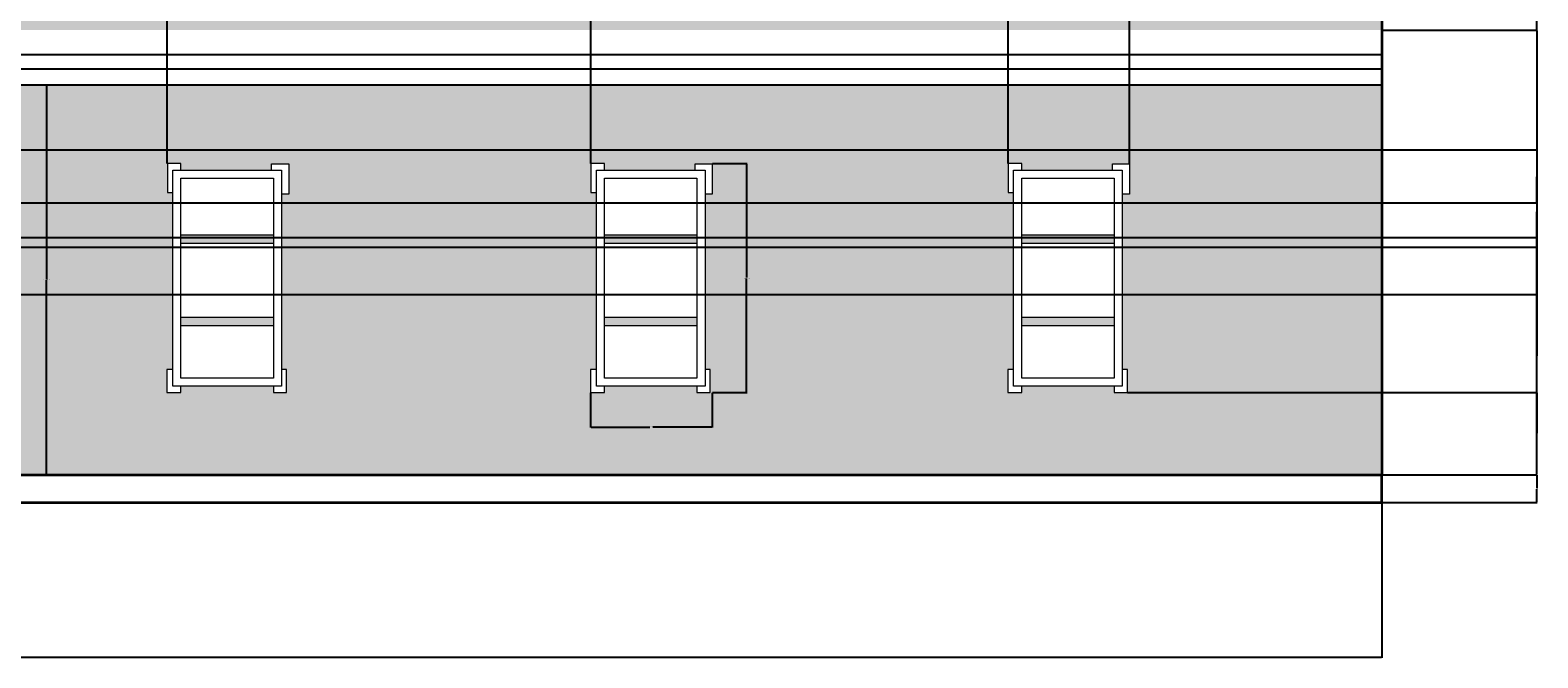
# Model space of a CAD drawing. Units: inches. Extents: x -46 to 1209, y 110 to 778.
# Tile 4 of 5: x 652 to 1209, y 110 to 342. Entities that reach past the tile are written whole.
import ezdxf

# ---------------------------------------------------------------- set-up
doc = ezdxf.new("R2010")
doc.units = ezdxf.units.IN
doc.header["$MEASUREMENT"] = 0
for name, color, linetype, lineweight in [('A-ANNO-DIMS', 2, 'Continuous', 18), ('A-ELEV-BASE', 7, 'Continuous', 35), ('A-GLAZ', 4, 'Continuous', 20), ('A-GLAZ-PATT', 9, 'Continuous', 13), ('A-WALL', 7, 'Continuous', 35), ('A-WALL-PATT', 252, 'Continuous', 13), ('A-WALL-TRIM', 42, 'Continuous', 25)]:
    doc.layers.add(name, color=color, linetype=linetype, lineweight=lineweight)
doc.styles.get("Standard").update_dxf_attribs({"font": 'arial.ttf'})
doc.dimstyles.get("Standard").update_dxf_attribs({"dimtxt": 0.18, "dimasz": 0.18, "dimexe": 0.18, "dimexo": 0.0625, "dimgap": 0.09, "dimtad": 0, "dimtih": 1, "dimtoh": 1, "dimdec": 4, "dimzin": 0, "dimdsep": 46, "dimtxsty": 'Standard', "dimcen": 0.09, "dimadec": 0, "dimazin": 0, "dimtfac": 1, "dimtdec": 4, "dimtofl": 0, "dimtmove": 0, "dimatfit": 3, "dimfxl": 1, "dimtolj": 1, "dimtzin": 0, "dimarcsym": 0})

# ---------------------------------------------------------------- blocks, each defined once
blk = doc.blocks.new('WIN-TALL-3-LIGHT')
for p, q in [((5.17, 84.79), (0.14, 84.79)), ((0.14, 84.79), (0.14, 74.08)), ((5.17, 82.37), (5.17, 84.79)), ((38.71, 82.37), (38.71, 84.69)), ((38.71, 84.69), (45.05, 84.69)), ((45.05, 84.69), (45.05, 73.44)), ((0.14, 74.08), (2.17, 74.08)), ((45.05, 73.44), (42.37, 73.44)), ((5.17, 58.36), (39.37, 58.36)), ((5.17, 55.27), (39.37, 55.27)), ((5.17, 27.98), (39.37, 27.98)), ((5.17, 24.89), (39.37, 24.89)), ((2.17, 8.6), (0, 8.6)), ((0, 8.6), (0, 0)), ((44.29, 8.6), (42.37, 8.6)), ((44.29, 0.11), (44.29, 8.6)), ((0, 0), (5.17, 0)), ((5.17, 0), (5.17, 2.36)), ((39.37, 2.36), (39.37, 0.11)), ((39.37, 0.11), (44.29, 0.11))]:
    blk.add_line(p, q)
for points in [[(2.17, 82.37), (42.37, 82.37), (42.37, 2.36), (2.17, 2.36)], [(5.17, 79.37), (39.37, 79.37), (39.37, 5.36), (5.17, 5.36)]]:
    blk.add_lwpolyline(points, close=True)
blk = doc.blocks.new('*D16')
at = {"layer": 'A-ANNO-DIMS', "color": 0, "lineweight": -2, "transparency": 16777216}
for p, q in [((904.03, 292.89), (916.87, 292.89)), ((916.69, 292.71), (916.69, 250.68)), ((916.69, 208.28), (916.69, 250.31)), ((904.03, 208.1), (916.87, 208.1))]:
    blk.add_line(p, q, dxfattribs=at)
at = {"layer": 'A-ANNO-DIMS', "color": 0, "transparency": 16777216}
for points in [[(916.66, 292.71), (916.72, 292.71), (916.69, 292.89)], [(916.66, 208.28), (916.72, 208.28), (916.69, 208.1)]]:
    blk.add_solid(points, dxfattribs=at)
at = {"layer": 'Defpoints', "color": 0, "transparency": 16777216}
for p in [(903.97, 292.89), (916.69, 292.89), (903.97, 208.1)]:
    blk.add_point(p, dxfattribs=at)
at = {"layer": 'A-ANNO-DIMS', "color": 0, "transparency": 16777216, "insert": (916.69, 250.5), "char_height": 0.18, "attachment_point": 5}
blk.add_mtext('\\A1;THREE-LIGHT WINDOW 85 TYP.', dxfattribs=at)
blk = doc.blocks.new('*D17')
at = {"layer": 'A-ANNO-DIMS', "color": 0, "lineweight": -2, "transparency": 16777216}
for p, q in [((858.92, 208.04), (858.92, 195.2)), ((903.97, 208.04), (903.97, 195.2)), ((859.1, 195.38), (880.91, 195.38)), ((903.79, 195.38), (881.98, 195.38))]:
    blk.add_line(p, q, dxfattribs=at)
at = {"layer": 'A-ANNO-DIMS', "color": 0, "transparency": 16777216}
for points in [[(859.1, 195.41), (859.1, 195.35), (858.92, 195.38)], [(903.79, 195.41), (903.79, 195.35), (903.97, 195.38)]]:
    blk.add_solid(points, dxfattribs=at)
at = {"layer": 'Defpoints', "color": 0, "transparency": 16777216}
for p in [(858.92, 208.1), (903.97, 208.1), (903.97, 195.38)]:
    blk.add_point(p, dxfattribs=at)
at = {"layer": 'A-ANNO-DIMS', "color": 0, "transparency": 16777216, "insert": (881.45, 195.38), "char_height": 0.18, "attachment_point": 5}
blk.add_mtext('\\A1;45 TYP.', dxfattribs=at)
blk = doc.blocks.new('*D22')
at = {"layer": 'A-ANNO-DIMS', "color": 0, "lineweight": -2, "transparency": 16777216}
for p, q in [((635.97, 321.99), (657.72, 321.99)), ((657.54, 321.81), (657.54, 250.04)), ((657.54, 177.91), (657.54, 249.68)), ((635.97, 177.73), (657.72, 177.73))]:
    blk.add_line(p, q, dxfattribs=at)
at = {"layer": 'A-ANNO-DIMS', "color": 0, "transparency": 16777216}
for points in [[(657.51, 321.81), (657.57, 321.81), (657.54, 321.99)], [(657.51, 177.91), (657.57, 177.91), (657.54, 177.73)]]:
    blk.add_solid(points, dxfattribs=at)
at = {"layer": 'Defpoints', "color": 0, "transparency": 16777216}
for p in [(635.91, 321.99), (657.54, 321.99), (635.91, 177.73)]:
    blk.add_point(p, dxfattribs=at)
at = {"layer": 'A-ANNO-DIMS', "color": 0, "transparency": 16777216, "insert": (657.54, 249.86), "char_height": 0.18, "attachment_point": 5}
blk.add_mtext('\\A1;ENTRY COLUMN 144 TYP.', dxfattribs=at)
blk = doc.blocks.new('*D28')
at = {"layer": 'A-ANNO-DIMS', "color": 0, "lineweight": -2, "transparency": 16777216}
for p, q in [((11.98, 329.67), (11.98, 109.96)), ((1151.8, 167.37), (1151.8, 109.96)), ((12.16, 110.14), (581.44, 110.14)), ((1151.62, 110.14), (582.35, 110.14))]:
    blk.add_line(p, q, dxfattribs=at)
at = {"layer": 'A-ANNO-DIMS', "color": 0, "transparency": 16777216}
for points in [[(12.16, 110.17), (12.16, 110.11), (11.98, 110.14)], [(1151.62, 110.17), (1151.62, 110.11), (1151.8, 110.14)]]:
    blk.add_solid(points, dxfattribs=at)
at = {"layer": 'Defpoints', "color": 0, "transparency": 16777216}
for p in [(11.98, 329.73), (1151.8, 167.44), (1151.8, 110.14)]:
    blk.add_point(p, dxfattribs=at)
at = {"layer": 'A-ANNO-DIMS', "color": 0, "transparency": 16777216, "insert": (581.89, 110.14), "char_height": 0.18, "attachment_point": 5}
blk.add_mtext('\\A1;1139.8', dxfattribs=at)
blk = doc.blocks.new('*D35')
at = {"layer": 'A-ANNO-DIMS', "color": 0, "lineweight": -2, "transparency": 16777216}
for p, q in [((368.5, 278.33), (1209.28, 278.33)), ((1209.1, 278.15), (1209.1, 228.21)), ((1209.1, 177.91), (1209.1, 227.85)), ((368.5, 177.73), (1209.28, 177.73))]:
    blk.add_line(p, q, dxfattribs=at)
at = {"layer": 'A-ANNO-DIMS', "color": 0, "transparency": 16777216}
for points in [[(1209.07, 278.15), (1209.13, 278.15), (1209.1, 278.33)], [(1209.07, 177.91), (1209.13, 177.91), (1209.1, 177.73)]]:
    blk.add_solid(points, dxfattribs=at)
at = {"layer": 'Defpoints', "color": 0, "transparency": 16777216}
for p in [(368.44, 278.33), (1209.1, 278.33), (368.44, 177.73)]:
    blk.add_point(p, dxfattribs=at)
at = {"layer": 'A-ANNO-DIMS', "color": 0, "transparency": 16777216, "insert": (1209.1, 228.03), "char_height": 0.18, "attachment_point": 5}
blk.add_mtext('\\A1;100.6', dxfattribs=at)
blk = doc.blocks.new('*D36')
at = {"layer": 'A-ANNO-DIMS', "color": 0, "lineweight": -2, "transparency": 16777216}
for p, q in [((310.94, 297.96), (1209.28, 297.96)), ((1209.1, 297.78), (1209.1, 288.33)), ((1209.1, 278.51), (1209.1, 287.96)), ((368.5, 278.33), (1209.28, 278.33))]:
    blk.add_line(p, q, dxfattribs=at)
at = {"layer": 'A-ANNO-DIMS', "color": 0, "transparency": 16777216}
for points in [[(1209.07, 297.78), (1209.13, 297.78), (1209.1, 297.96)], [(1209.07, 278.51), (1209.13, 278.51), (1209.1, 278.33)]]:
    blk.add_solid(points, dxfattribs=at)
at = {"layer": 'Defpoints', "color": 0, "transparency": 16777216}
for p in [(310.88, 297.96), (1209.1, 297.96), (368.44, 278.33)]:
    blk.add_point(p, dxfattribs=at)
at = {"layer": 'A-ANNO-DIMS', "color": 0, "transparency": 16777216, "insert": (1209.1, 288.14), "char_height": 0.18, "attachment_point": 5}
blk.add_mtext('\\A1;19.63', dxfattribs=at)
blk = doc.blocks.new('*D41')
at = {"layer": 'A-ANNO-DIMS', "color": 0, "lineweight": -2, "transparency": 16777216}
for p, q in [((198.93, 261.94), (1209.28, 261.94)), ((1209.1, 261.76), (1209.1, 253.4)), ((1209.1, 244.67), (1209.1, 253.04)), ((198.93, 244.49), (1209.28, 244.49))]:
    blk.add_line(p, q, dxfattribs=at)
at = {"layer": 'A-ANNO-DIMS', "color": 0, "transparency": 16777216}
for points in [[(1209.07, 261.76), (1209.13, 261.76), (1209.1, 261.94)], [(1209.07, 244.67), (1209.13, 244.67), (1209.1, 244.49)]]:
    blk.add_solid(points, dxfattribs=at)
at = {"layer": 'Defpoints', "color": 0, "transparency": 16777216}
for p in [(198.86, 261.94), (1209.1, 261.94), (198.86, 244.49)]:
    blk.add_point(p, dxfattribs=at)
at = {"layer": 'A-ANNO-DIMS', "color": 0, "transparency": 16777216, "insert": (1209.1, 253.22), "char_height": 0.18, "attachment_point": 5}
blk.add_mtext('\\A1;17.446', dxfattribs=at)
blk = doc.blocks.new('*D44')
at = {"layer": 'A-ANNO-DIMS', "color": 0, "lineweight": -2, "transparency": 16777216}
for p, q in [((18.95, 265.48), (1209.28, 265.48)), ((1209.1, 265.3), (1209.1, 221.79)), ((1209.1, 177.91), (1209.1, 221.42)), ((15.29, 177.73), (1209.28, 177.73))]:
    blk.add_line(p, q, dxfattribs=at)
at = {"layer": 'A-ANNO-DIMS', "color": 0, "transparency": 16777216}
for points in [[(1209.07, 265.3), (1209.13, 265.3), (1209.1, 265.48)], [(1209.07, 177.91), (1209.13, 177.91), (1209.1, 177.73)]]:
    blk.add_solid(points, dxfattribs=at)
at = {"layer": 'Defpoints', "color": 0, "transparency": 16777216}
for p in [(18.89, 265.48), (1209.1, 265.48), (15.23, 177.73)]:
    blk.add_point(p, dxfattribs=at)
at = {"layer": 'A-ANNO-DIMS', "color": 0, "transparency": 16777216, "insert": (1209.1, 221.6), "char_height": 0.18, "attachment_point": 5}
blk.add_mtext('\\A1;87.74', dxfattribs=at)
blk = doc.blocks.new('*D53')
at = {"layer": 'A-ANNO-DIMS', "color": 0, "lineweight": -2, "transparency": 16777216}
for p, q in [((1151.86, 177.73), (1209.28, 177.73)), ((1209.1, 177.55), (1209.1, 172.77)), ((1151.86, 167.44), (1209.28, 167.44)), ((1209.1, 167.62), (1209.1, 172.4))]:
    blk.add_line(p, q, dxfattribs=at)
at = {"layer": 'A-ANNO-DIMS', "color": 0, "transparency": 16777216}
for points in [[(1209.07, 177.55), (1209.13, 177.55), (1209.1, 177.73)], [(1209.07, 167.62), (1209.13, 167.62), (1209.1, 167.44)]]:
    blk.add_solid(points, dxfattribs=at)
at = {"layer": 'Defpoints', "color": 0, "transparency": 16777216}
for p in [(1151.8, 177.73), (1209.1, 177.73), (1151.8, 167.44)]:
    blk.add_point(p, dxfattribs=at)
at = {"layer": 'A-ANNO-DIMS', "color": 0, "transparency": 16777216, "insert": (1209.1, 172.58), "char_height": 0.18, "attachment_point": 5}
blk.add_mtext('\\A1;10.297', dxfattribs=at)
blk = doc.blocks.new('*D54')
at = {"layer": 'A-ANNO-DIMS', "color": 0, "lineweight": -2, "transparency": 16777216}
for p, q in [((1057.66, 208.21), (1209.28, 208.21)), ((1209.1, 208.03), (1209.1, 193.15)), ((1209.1, 177.91), (1209.1, 192.79)), ((1151.86, 177.73), (1209.28, 177.73))]:
    blk.add_line(p, q, dxfattribs=at)
at = {"layer": 'A-ANNO-DIMS', "color": 0, "transparency": 16777216}
for points in [[(1209.07, 208.03), (1209.13, 208.03), (1209.1, 208.21)], [(1209.07, 177.91), (1209.13, 177.91), (1209.1, 177.73)]]:
    blk.add_solid(points, dxfattribs=at)
at = {"layer": 'Defpoints', "color": 0, "transparency": 16777216}
for p in [(1057.6, 208.21), (1209.1, 208.21), (1151.8, 177.73)]:
    blk.add_point(p, dxfattribs=at)
at = {"layer": 'A-ANNO-DIMS', "color": 0, "transparency": 16777216, "insert": (1209.1, 192.97), "char_height": 0.18, "attachment_point": 5}
blk.add_mtext('\\A1;30.48', dxfattribs=at)
blk = doc.blocks.new('*D55')
at = {"layer": 'A-ANNO-DIMS', "color": 0, "lineweight": -2, "transparency": 16777216}
for p, q in [((1151.86, 342.26), (1209.28, 342.26)), ((1209.1, 342.08), (1209.1, 275.42)), ((1209.1, 208.39), (1209.1, 275.05)), ((1057.66, 208.21), (1209.28, 208.21))]:
    blk.add_line(p, q, dxfattribs=at)
at = {"layer": 'A-ANNO-DIMS', "color": 0, "transparency": 16777216}
for points in [[(1209.07, 342.08), (1209.13, 342.08), (1209.1, 342.26)], [(1209.07, 208.39), (1209.13, 208.39), (1209.1, 208.21)]]:
    blk.add_solid(points, dxfattribs=at)
at = {"layer": 'Defpoints', "color": 0, "transparency": 16777216}
for p in [(1151.8, 342.26), (1209.1, 342.26), (1057.6, 208.21)]:
    blk.add_point(p, dxfattribs=at)
at = {"layer": 'A-ANNO-DIMS', "color": 0, "transparency": 16777216, "insert": (1209.1, 275.24), "char_height": 0.18, "attachment_point": 5}
blk.add_mtext('\\A1;134.05', dxfattribs=at)
blk = doc.blocks.new('*D56')
at = {"layer": 'A-ANNO-DIMS', "color": 0, "lineweight": -2, "transparency": 16777216}
for p, q in [((1078.14, 455.08), (1209.28, 455.08)), ((1209.1, 454.9), (1209.1, 398.86)), ((1209.1, 342.44), (1209.1, 398.49)), ((1151.86, 342.26), (1209.28, 342.26))]:
    blk.add_line(p, q, dxfattribs=at)
at = {"layer": 'A-ANNO-DIMS', "color": 0, "transparency": 16777216}
for points in [[(1209.07, 454.9), (1209.13, 454.9), (1209.1, 455.08)], [(1209.07, 342.44), (1209.13, 342.44), (1209.1, 342.26)]]:
    blk.add_solid(points, dxfattribs=at)
at = {"layer": 'Defpoints', "color": 0, "transparency": 16777216}
for p in [(1078.08, 455.08), (1209.1, 455.08), (1151.8, 342.26)]:
    blk.add_point(p, dxfattribs=at)
at = {"layer": 'A-ANNO-DIMS', "color": 0, "transparency": 16777216, "insert": (1209.1, 398.67), "char_height": 0.18, "attachment_point": 5}
blk.add_mtext('\\A1;112.82', dxfattribs=at)
blk = doc.blocks.new('*D71')
at = {"layer": 'A-ANNO-DIMS', "color": 0, "lineweight": -2, "transparency": 16777216}
for p, q in [((702.3, 292.96), (702.3, 777.55)), ((702.48, 777.37), (780.23, 777.37)), ((858.88, 777.37), (781.14, 777.37)), ((859.06, 292.96), (859.06, 777.55))]:
    blk.add_line(p, q, dxfattribs=at)
at = {"layer": 'A-ANNO-DIMS', "color": 0, "transparency": 16777216}
for points in [[(702.48, 777.4), (702.48, 777.34), (702.3, 777.37)], [(858.88, 777.4), (858.88, 777.34), (859.06, 777.37)]]:
    blk.add_solid(points, dxfattribs=at)
at = {"layer": 'Defpoints', "color": 0, "transparency": 16777216}
for p in [(859.06, 777.37), (702.3, 292.89), (859.06, 292.89)]:
    blk.add_point(p, dxfattribs=at)
at = {"layer": 'A-ANNO-DIMS', "color": 0, "transparency": 16777216, "insert": (780.68, 777.37), "char_height": 0.18, "attachment_point": 5}
blk.add_mtext('\\A1;156.76', dxfattribs=at)
blk = doc.blocks.new('*D72')
at = {"layer": 'A-ANNO-DIMS', "color": 0, "lineweight": -2, "transparency": 16777216}
for p, q in [((859.06, 292.96), (859.06, 777.55)), ((859.24, 777.37), (935.87, 777.37)), ((1013.27, 777.37), (936.64, 777.37)), ((1013.45, 292.96), (1013.45, 777.55))]:
    blk.add_line(p, q, dxfattribs=at)
at = {"layer": 'A-ANNO-DIMS', "color": 0, "transparency": 16777216}
for points in [[(859.24, 777.4), (859.24, 777.34), (859.06, 777.37)], [(1013.27, 777.4), (1013.27, 777.34), (1013.45, 777.37)]]:
    blk.add_solid(points, dxfattribs=at)
at = {"layer": 'Defpoints', "color": 0, "transparency": 16777216}
for p in [(1013.45, 777.37), (859.06, 292.89), (1013.45, 292.89)]:
    blk.add_point(p, dxfattribs=at)
at = {"layer": 'A-ANNO-DIMS', "color": 0, "transparency": 16777216, "insert": (936.26, 777.37), "char_height": 0.18, "attachment_point": 5}
blk.add_mtext('\\A1;154.4', dxfattribs=at)
blk = doc.blocks.new('*D73')
at = {"layer": 'A-ANNO-DIMS', "color": 0, "lineweight": -2, "transparency": 16777216}
for p, q in [((1058.36, 292.85), (1058.36, 777.55)), ((1058.54, 777.37), (1104.69, 777.37)), ((1151.62, 777.37), (1105.47, 777.37)), ((1151.8, 322.05), (1151.8, 777.55))]:
    blk.add_line(p, q, dxfattribs=at)
at = {"layer": 'A-ANNO-DIMS', "color": 0, "transparency": 16777216}
for points in [[(1058.54, 777.4), (1058.54, 777.34), (1058.36, 777.37)], [(1151.62, 777.4), (1151.62, 777.34), (1151.8, 777.37)]]:
    blk.add_solid(points, dxfattribs=at)
at = {"layer": 'Defpoints', "color": 0, "transparency": 16777216}
for p in [(1151.8, 777.37), (1151.8, 321.99), (1058.36, 292.79)]:
    blk.add_point(p, dxfattribs=at)
at = {"layer": 'A-ANNO-DIMS', "color": 0, "transparency": 16777216, "insert": (1105.08, 777.37), "char_height": 0.18, "attachment_point": 5}
blk.add_mtext('\\A1;93.44', dxfattribs=at)

msp = doc.modelspace()

# ---------------------------------------------------------------- hatches: boundary and pattern name
at = {"layer": 'A-GLAZ-PATT'}
h = msp.add_hatch(color=256, dxfattribs=at)
h.dxf.hatch_style = 1
h.paths.add_polyline_path([(524.7711, 532.926), (523.2165, 532.926), (521.7711, 532.926), (521.7711, 499.4601), (524.7711, 499.4601)])
h.paths.add_polyline_path([(524.7711, 499.4601), (521.7711, 499.4601), (521.7711, 496.0287), (524.7711, 496.0287)])
h.paths.add_polyline_path([(568.2834, 499.4601), (524.7711, 499.4601), (524.7711, 496.0287), (568.2834, 496.0287)])
h.paths.add_polyline_path([(521.7711, 499.4601), (483.2375, 499.4601), (483.2375, 496.0287), (521.7711, 496.0287)])
h.paths.add_polyline_path([(524.7711, 496.0287), (521.7711, 496.0287), (521.7711, 425.5857), (524.7711, 425.5857)])
h.paths.add_polyline_path([(568.2834, 457.8123), (524.7711, 457.8123), (524.7711, 454.4649), (568.2834, 454.4649)])
h.paths.add_polyline_path([(521.7711, 457.8123), (483.2375, 457.8123), (483.2375, 454.4649), (521.7711, 454.4649)])
h.paths.add_polyline_path([(741.5274, 266.4582), (707.3294, 266.4582), (707.3294, 263.369), (741.5274, 263.369)])
h.paths.add_polyline_path([(741.5274, 236.0814), (707.3294, 236.0814), (707.3294, 232.9922), (741.5274, 232.9922)])
h.paths.add_polyline_path([(898.2871, 266.4582), (864.0892, 266.4582), (864.0892, 263.369), (898.2871, 263.369)])
h.paths.add_polyline_path([(898.2871, 236.0814), (864.0892, 236.0814), (864.0892, 232.9922), (898.2871, 232.9922)])
h.paths.add_polyline_path([(1052.6765, 266.4582), (1018.4786, 266.4582), (1018.4786, 263.369), (1052.6765, 263.369)])
h.paths.add_polyline_path([(1052.6765, 236.0814), (1018.4786, 236.0814), (1018.4786, 232.9922), (1052.6765, 232.9922)])
at = {"layer": 'A-WALL-PATT'}
h = msp.add_hatch(dxfattribs=at)
h.set_pattern_fill('AR-CONC', color=256, scale=3)
h.paths.add_polyline_path([(387.8322, 595.7911), (179.1007, 595.7911), (179.1007, 451.7911), (179.1007, 439.7911), (220.892, 454.7186), (313.6366, 436.1845), (387.8322, 376.346)])
h.paths.add_polyline_path([(276.7646, 548.5945), (292.8821, 548.5945), (292.8821, 553.0308), (295.9402, 553.0308), (295.9402, 548.5945), (313.3682, 548.5945), (313.3682, 512.6263), (276.7646, 512.6263)], flags=16)
h.paths.add_polyline_path([(278.6627, 545.0233), (312.1316, 545.0233), (312.1316, 514.6792), (278.6627, 514.6792)], flags=0)
h.paths.add_polyline_path([(326.2691, 548.5945), (341.5129, 548.5945), (341.5129, 553.0308), (344.571, 553.0308), (344.571, 548.5945), (362.8728, 548.5945), (362.8728, 512.6263), (326.2691, 512.6263)], flags=16)
h.paths.add_polyline_path([(328.1673, 545.0233), (361.6362, 545.0233), (361.6362, 514.6792), (328.1673, 514.6792)], flags=0)
h.paths.add_polyline_path([(651.5361, 595.7911), (415.401, 595.7911), (387.8322, 595.7911), (387.8322, 376.346), (409.6414, 342.2631), (651.5361, 342.2631)])
h.paths.add_polyline_path([(470.5081, 534.2042), (467.0793, 534.2042), (467.0793, 554.4029), (483.2058, 554.4029), (483.2058, 549.2024), (518.0634, 549.2024), (518.0634, 557.4852), (520.3257, 557.4852), (520.3257, 564.6435), (523.2165, 564.6435), (523.2165, 557.4852), (525.4788, 557.4852), (525.4788, 549.2024), (567.4184, 549.2024), (567.4184, 554.4029), (579.1691, 554.4029), (579.1691, 534.2042), (575.9249, 534.2042), (575.9249, 428.1662), (580.259, 428.1662), (580.259, 412.8567), (567.4184, 412.8567), (567.4184, 417.1318), (483.8186, 417.1318), (483.8186, 413.5449), (465.7589, 413.5449), (465.7589, 426.3336), (470.5081, 426.3336)], flags=16)
h.paths.add_polyline_path([(483.2375, 532.926), (568.2834, 532.926), (568.2834, 425.5857), (483.2375, 425.5857)], flags=0)
h.paths.add_polyline_path([(431.7717, 578.8147), (431.7717, 585.9699), (440.9467, 585.9699), (440.9467, 578.8147)], flags=16)
h.paths.add_polyline_path([(423.2681, 578.8147), (414.0931, 578.8147), (414.0931, 585.9699), (423.2681, 585.9699)], flags=16)
h.paths.add_polyline_path([(447.8839, 578.8147), (447.8839, 585.9699), (457.0589, 585.9699), (457.0589, 578.8147)], flags=16)
h.paths.add_polyline_path([(406.5964, 578.8147), (397.4214, 578.8147), (397.4214, 585.9699), (406.5964, 585.9699)], flags=16)
h.paths.add_polyline_path([(466.0101, 578.8147), (466.0101, 585.9699), (475.1851, 585.9699), (475.1851, 578.8147)], flags=16)
h.paths.add_polyline_path([(483.6888, 578.8147), (483.6888, 585.9699), (492.8638, 585.9699), (492.8638, 578.8147)], flags=16)
h.paths.add_polyline_path([(504.0528, 578.8147), (504.0528, 585.9699), (513.2278, 585.9699), (513.2278, 578.8147)], flags=16)
h.paths.add_polyline_path([(523.0742, 578.8147), (523.0742, 585.9699), (532.2492, 585.9699), (532.2492, 578.8147)], flags=16)
h.paths.add_polyline_path([(542.3193, 578.8147), (542.3193, 585.9699), (551.4943, 585.9699), (551.4943, 578.8147)], flags=16)
h.paths.add_polyline_path([(559.998, 578.8147), (559.998, 585.9699), (569.1729, 585.9699), (569.1729, 578.8147)], flags=16)
h.paths.add_polyline_path([(580.1382, 578.8147), (580.1382, 585.9699), (589.3132, 585.9699), (589.3132, 578.8147)], flags=16)
h.paths.add_polyline_path([(598.3313, 578.8147), (598.3313, 585.9699), (607.5063, 585.9699), (607.5063, 578.8147)], flags=16)
h.paths.add_polyline_path([(618.2477, 578.8147), (618.2477, 585.9699), (627.4227, 585.9699), (627.4227, 578.8147)], flags=16)
h.paths.add_polyline_path([(636.8215, 578.8147), (636.8215, 585.9699), (645.9965, 585.9699), (645.9965, 578.8147)], flags=16)
h.paths.add_polyline_path([(1151.8016, 595.7911), (651.5361, 595.7911), (651.5361, 342.2631), (939.9139, 342.2631), (1151.8016, 342.2631)])
h.paths.add_polyline_path([(683.9631, 455.0835), (683.9631, 537.4823), (720.8864, 537.4823), (720.8864, 547.6453), (727.8922, 547.6453), (727.8922, 537.4823), (767.8177, 537.4823), (767.8177, 455.0835)], flags=16)
h.paths.add_polyline_path([(688.3115, 459.7865), (688.3115, 529.3012), (764.9847, 529.3012), (764.9847, 459.7865)], flags=0)
h.paths.add_polyline_path([(840.5045, 455.0835), (840.5045, 537.4823), (877.4279, 537.4823), (877.4279, 547.6453), (884.4336, 547.6453), (884.4336, 537.4823), (924.3592, 537.4823), (924.3592, 455.0835)], flags=16)
h.paths.add_polyline_path([(844.853, 459.7865), (844.853, 529.3012), (921.5262, 529.3012), (921.5262, 459.7865)], flags=0)
h.paths.add_polyline_path([(994.2223, 455.0835), (994.2223, 537.4823), (1031.1457, 537.4823), (1031.1457, 547.6453), (1038.1514, 547.6453), (1038.1514, 537.4823), (1078.077, 537.4823), (1078.077, 455.0835)], flags=16)
h.paths.add_polyline_path([(998.5708, 459.7865), (998.5708, 529.3012), (1075.244, 529.3012), (1075.244, 459.7865)], flags=0)
h.paths.add_polyline_path([(1151.8016, 321.9907), (941.4829, 321.9907), (632.1261, 321.9907), (632.1261, 313.1625), (629.6322, 313.1625), (629.6322, 281.6236), (635.9059, 281.6236), (635.9059, 276.2471), (629.6322, 276.2471), (629.6322, 185.3878), (632.1261, 185.3878), (632.1261, 177.7316), (1151.8016, 177.7316)])
h.paths.add_polyline_path([(704.3294, 282.1806), (702.3037, 282.1806), (702.3037, 292.8947), (707.3294, 292.8947), (707.3294, 290.4743), (740.8704, 290.4743), (740.8704, 292.7856), (747.2108, 292.7856), (747.2108, 281.5404), (744.5274, 281.5404), (744.5274, 216.7007), (746.4513, 216.7007), (746.4513, 208.2103), (741.5274, 208.2103), (741.5274, 210.4615), (707.3294, 210.4615), (707.3294, 208.0997), (702.1613, 208.0997), (702.1613, 216.7007), (704.3294, 216.7007)], flags=16)
h.paths.add_polyline_path([(707.3294, 287.4743), (741.5274, 287.4743), (741.5274, 213.4615), (707.3294, 213.4615)], flags=0)
h.paths.add_polyline_path([(859.0635, 282.1806), (859.0635, 292.8947), (864.0892, 292.8947), (864.0892, 290.4743), (897.6301, 290.4743), (897.6301, 292.7856), (903.9705, 292.7856), (903.9705, 281.5404), (901.2871, 281.5404), (901.2871, 216.7007), (903.2111, 216.7007), (903.2111, 208.2103), (898.2871, 208.2103), (898.2871, 210.4615), (864.0892, 210.4615), (864.0892, 208.0997), (858.9211, 208.0997), (858.9211, 216.7007), (861.0892, 216.7007), (861.0892, 282.1806)], flags=16)
h.paths.add_polyline_path([(864.0892, 287.4743), (898.2871, 287.4743), (898.2871, 213.4615), (864.0892, 213.4615)], flags=0)
h.paths.add_polyline_path([(1013.4529, 282.1806), (1013.4529, 292.8947), (1018.4786, 292.8947), (1018.4786, 290.4743), (1052.0195, 290.4743), (1052.0195, 292.7856), (1058.3599, 292.7856), (1058.3599, 281.5404), (1055.6765, 281.5404), (1055.6765, 216.7007), (1057.6005, 216.7007), (1057.6005, 208.2103), (1052.6765, 208.2103), (1052.6765, 210.4615), (1018.4786, 210.4615), (1018.4786, 208.0997), (1013.3105, 208.0997), (1013.3105, 216.7007), (1015.4786, 216.7007), (1015.4786, 282.1806)], flags=16)
h.paths.add_polyline_path([(1018.4786, 287.4743), (1052.6765, 287.4743), (1052.6765, 213.4615), (1018.4786, 213.4615)], flags=0)
h.paths.add_polyline_path([(431.9367, 276.2471), (423.7231, 276.2471), (423.7231, 281.6236), (431.9367, 281.6236), (431.9367, 313.1625), (430.3199, 313.1625), (430.3199, 321.9907), (406.6462, 321.9907), (406.6462, 321.7316), (405.6256, 177.7316), (430.3199, 177.7316), (430.3199, 185.3878), (431.9367, 185.3878)])
h.paths.add_polyline_path([(406.6462, 321.7316), (406.6462, 321.9907), (363.2774, 321.9907), (58.5947, 321.7316), (57.7764, 206.2827), (87.7834, 206.0701), (87.7834, 290.4607), (89.9075, 293.33), (149.9611, 311.663), (149.9611, 316.8909), (153.3383, 316.8909), (153.3383, 311.1504), (213.2336, 293.3362), (215.3783, 290.4607), (215.3783, 205.1657), (246.588, 204.9445), (246.588, 290.0127), (248.7121, 292.882), (308.2509, 311.0579), (308.2509, 316.0122), (311.6281, 316.0122), (311.6281, 310.8556), (372.0381, 292.8882), (374.1829, 290.0127), (374.1829, 204.0402), (405.8105, 203.8161)])
h.paths.add_polyline_path([(333, 359.5), (292.5, 377), (250.5, 387.5), (199, 387.5), (155, 377.5), (123.5, 364), (101.4287, 342.2631), (363.2774, 342.2631)])
h.paths.add_polyline_path([(579.9721, 681.6773), (549.8011, 690.7996), (524.9646, 691.17), (482.8908, 691.7975), (447.0968, 679.2482), (416.3264, 659.1694), (597.1807, 659.1694)])

# ---------------------------------------------------------------- linework, layer by layer
at = {"layer": 'A-ELEV-BASE'}
for p, q in [((15.2259, 177.7316), (1151.8016, 177.7316)), ((1151.8016, 167.435), (1151.8016, 177.7316)), ((15.2259, 167.435), (1151.8016, 167.435))]:
    msp.add_line(p, q, dxfattribs=at)
at = {"layer": 'A-WALL'}
msp.add_line((1151.8016, 595.7911), (1151.8016, 177.7316), dxfattribs=at)
at = {"layer": 'A-WALL-TRIM'}
for p, q in [((415.401, 333.2621), (933.8719, 333.2621)), ((933.8719, 333.2621), (1151.8016, 333.2621)), ((406.6888, 327.9907), (918.2932, 327.9907)), ((918.2932, 327.9907), (1151.8016, 327.9907)), ((406.6462, 321.9907), (941.4829, 321.9907)), ((941.4829, 321.9907), (1151.8016, 321.9907))]:
    msp.add_line(p, q, dxfattribs=at)

# ---------------------------------------------------------------- block references
at = {"layer": 'A-GLAZ'}
for p in [(702.1613, 208.0997), (858.9211, 208.0997), (1013.3105, 208.0997)]:
    msp.add_blockref('WIN-TALL-3-LIGHT', p, dxfattribs=at)

# ---------------------------------------------------------------- dimensions: what is measured, and where the dimension line sits
at = {"layer": 'A-ANNO-DIMS'}
for base, p1, p2, override, picture, middle in [((859.0635, 777.3699), (702.3037, 292.8947), (859.0635, 292.8947), {"dimdec": 2, "dimlfac": 1, "dimrnd": 0, "dimzin": 0, "dimdsep": 46, "dimlunit": 2}, '*D71', (780.6836, 777.3699)), ((1013.4529, 777.3699), (859.0635, 292.8947), (1013.4529, 292.8947), {"dimdec": 1, "dimlfac": 1, "dimrnd": 0, "dimzin": 0, "dimdsep": 46, "dimlunit": 2}, '*D72', (936.2582, 777.3699)), ((1151.8016, 777.3699), (1058.3599, 292.7856), (1151.8016, 321.9907), {"dimdec": 2, "dimlfac": 1, "dimrnd": 0, "dimzin": 0, "dimdsep": 46, "dimlunit": 2}, '*D73', (1105.0807, 777.3699)), ((1151.8016, 110.135), (11.9842, 329.7316), (1151.8016, 167.435), {"dimdec": 1, "dimlfac": 1, "dimrnd": 0, "dimzin": 0, "dimdsep": 46, "dimlunit": 2}, '*D28', (581.8929, 110.135))]:
    dim = msp.add_linear_dim(base=base, p1=p1, p2=p2, dimstyle='Standard', override=override, dxfattribs=at)
    dim.commit()
    dim.dimension.update_dxf_attribs({"geometry": picture, "text_midpoint": middle})
for base, p1, p2, override, picture, middle in [((1209.1016, 455.0835), (1151.8016, 342.2631), (1078.077, 455.0835), {"dimdec": 2, "dimlfac": 1, "dimrnd": 0, "dimzin": 0, "dimdsep": 46, "dimlunit": 2}, '*D56', (1209.1016, 398.6733)), ((1209.1016, 342.2631), (1057.6005, 208.2103), (1151.8016, 342.2631), {"dimdec": 2, "dimlfac": 1, "dimrnd": 0, "dimzin": 0, "dimdsep": 46, "dimlunit": 2}, '*D55', (1209.1016, 275.2367)), ((1209.1016, 297.9586), (368.4424, 278.3288), (310.8814, 297.9586), {"dimdec": 2, "dimlfac": 1, "dimrnd": 0, "dimzin": 0, "dimdsep": 46, "dimlunit": 2}, '*D36', (1209.1016, 288.1437)), ((1209.1016, 278.3288), (368.4424, 177.7316), (368.4424, 278.3288), {"dimdec": 1, "dimlfac": 1, "dimrnd": 0, "dimzin": 0, "dimdsep": 46, "dimlunit": 2}, '*D35', (1209.1016, 228.0302)), ((1209.1016, 265.4762), (15.2259, 177.7316), (18.8869, 265.4762), {"dimdec": 2, "dimlfac": 1, "dimrnd": 0, "dimzin": 0, "dimdsep": 46, "dimlunit": 2}, '*D44', (1209.1016, 221.6039)), ((1209.1016, 261.9412), (198.8637, 244.4949), (198.8637, 261.9412), {"dimdec": 3, "dimlfac": 1, "dimrnd": 0, "dimzin": 0, "dimdsep": 46, "dimlunit": 2}, '*D41', (1209.1016, 253.218)), ((1209.1016, 208.2103), (1151.8016, 177.7316), (1057.6005, 208.2103), {"dimdec": 2, "dimlfac": 1, "dimrnd": 0, "dimzin": 0, "dimdsep": 46, "dimlunit": 2}, '*D54', (1209.1016, 192.9709)), ((1209.1016, 177.7316), (1151.8016, 167.435), (1151.8016, 177.7316), {"dimdec": 3, "dimlfac": 1, "dimrnd": 0, "dimzin": 0, "dimdsep": 46, "dimlunit": 2}, '*D53', (1209.1016, 172.5833))]:
    dim = msp.add_linear_dim(base=base, p1=p1, p2=p2, angle=90, dimstyle='Standard', override=override, dxfattribs=at)
    dim.commit()
    dim.dimension.update_dxf_attribs({"geometry": picture, "text_midpoint": middle})
for base, p1, p2, text, picture, middle in [((657.5447, 321.9907), (635.9059, 177.7316), (635.9059, 321.9907), 'ENTRY COLUMN <> TYP.', '*D22', (657.5447, 249.8612)), ((916.6897, 292.8947), (903.9705, 208.0997), (903.9705, 292.8947), 'THREE-LIGHT WINDOW <> TYP.', '*D16', (916.6897, 250.4972))]:
    dim = msp.add_linear_dim(base=base, p1=p1, p2=p2, angle=90, text=text, dimstyle='Standard', override={"dimdec": 0, "dimlfac": 1, "dimrnd": 0, "dimzin": 0, "dimdsep": 46, "dimlunit": 2}, dxfattribs=at)
    dim.commit()
    dim.dimension.update_dxf_attribs({"geometry": picture, "text_midpoint": middle})
dim = msp.add_linear_dim(base=(903.9705, 195.3805), p1=(858.9211, 208.0997), p2=(903.9705, 208.0997), text='<> TYP.', dimstyle='Standard', override={"dimdec": 0, "dimlfac": 1, "dimrnd": 0, "dimzin": 0, "dimdsep": 46, "dimlunit": 2}, dxfattribs=at)
dim.commit()
dim.dimension.update_dxf_attribs({"geometry": '*D17', "text_midpoint": (881.4458, 195.3805)})

doc.saveas('drawing.dxf')
